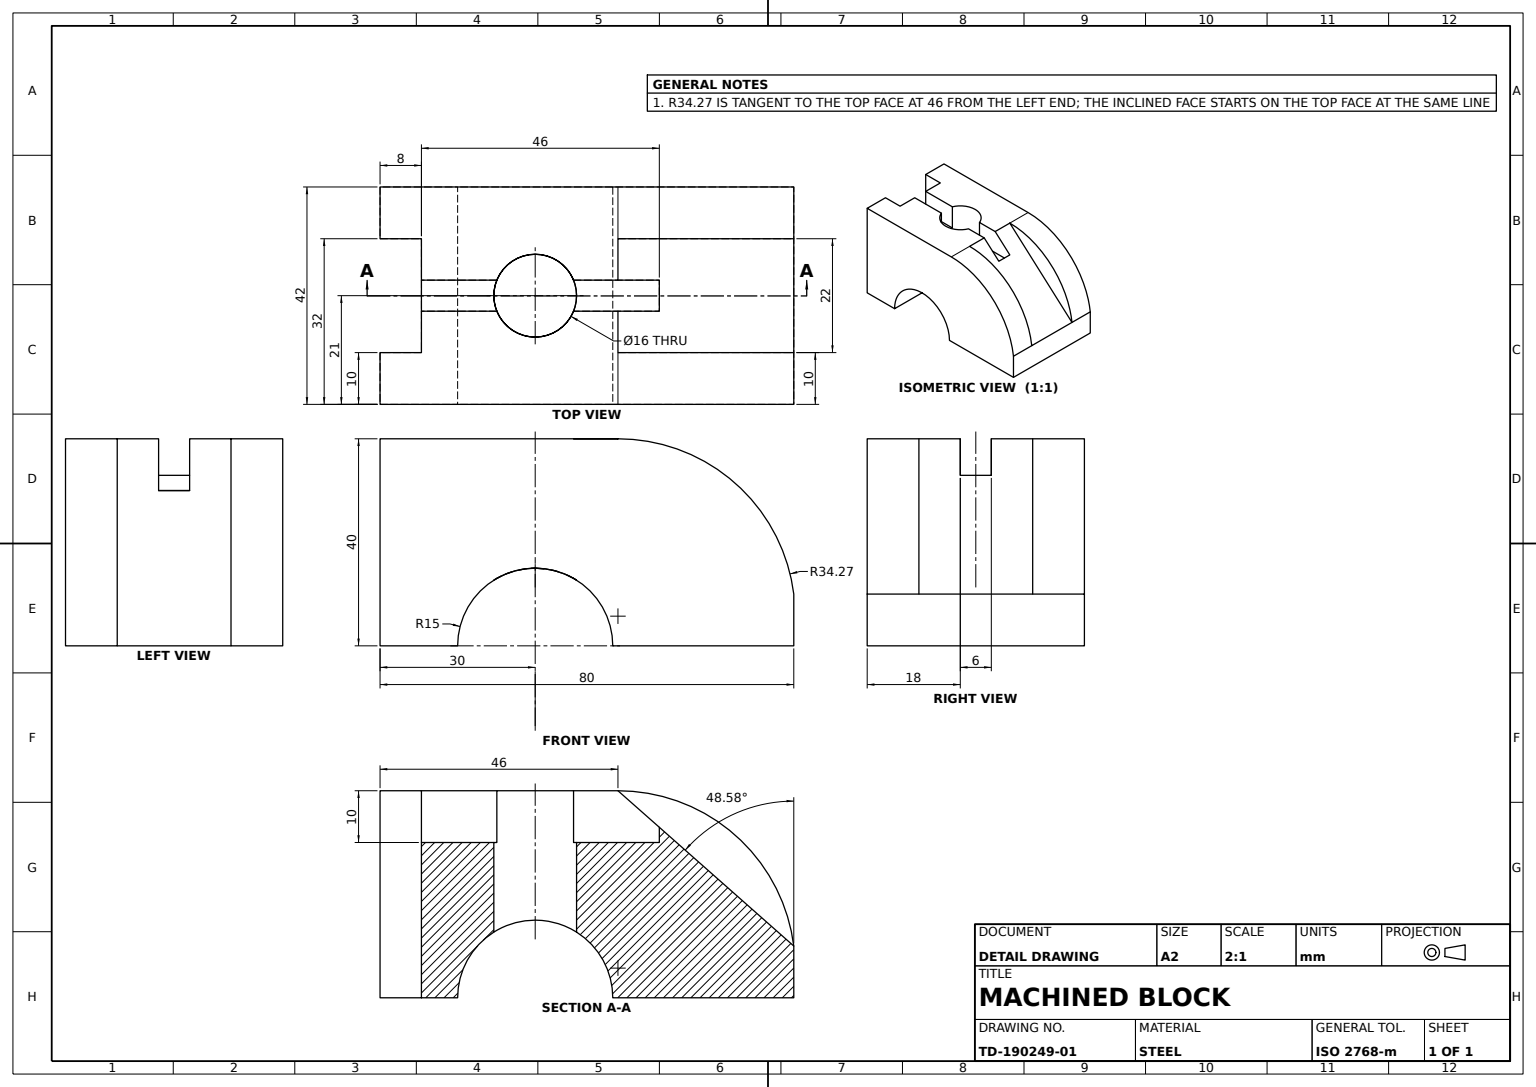
SolidWorks part; units mm, degrees
material "Plain Carbon Steel"
ref_plane "Front Plane" through (0, 0, 0) normal (0, 0, 1) x (1, 0, 0)
ref_plane "Top Plane" through (0, 0, 0) normal (0, 1, 0) x (1, 0, 0)
ref_plane "Right Plane" through (0, 0, 0) normal (1, 0, 0) x (0, 0, -1)
sketch "Base Block Profile" plane through (0, 0, 0) normal (0, 0, 1) x (1, 0, 0)
  line L0 (0, 0) -> (80, 0)
  line L1 (80, 0) -> (80, 40)
  line L2 (80, 40) -> (0, 40)
  line L3 (0, 40) -> (0, 0)
  dimension "D1" = 80
  dimension "D2" = 40
extrude "Base Block 80x40x42" add sketch "Base Block Profile" against normal blind 42
sketch "Top Slot Profile" plane through (0, 0, 0) normal (0, 0, 1) x (1, 0, 0)
  line L0 (0, 40) -> (0, 0) construction
  line L1 (46, 40) -> (46, 10)
  line L2 (80, 0) -> (80, 40) construction
  line L3 (46, 10) -> (80, 10)
  line L4 (0, 0) -> (80, 0) construction
  line L5 (80, 40) -> (0, 40) construction
  line L6 (46, 40) -> (80, 40)
  line L7 (80, 40) -> (80, 10)
  dimension "D1" = 46
  dimension "D2" = 10
extrude "Top Slot Cut 10" cut sketch "Top Slot Profile" against normal blind 10
sketch "Groove Profile" plane through (0, 0, -10) normal (0, 0, 1) x (1, 0, 0)
  line L0 (46, 40) -> (80, 10)
  line L1 (80, 10) -> (80, 40)
  line L2 (80, 40) -> (46, 40)
extrude "Groove Cut 22" cut sketch "Groove Profile" against normal blind 22
sketch "Groove Infill Profile" plane through (0, 0, 0) normal (0, 0, 1) x (1, 0, 0)
  line L0 (46, 40) -> (0, 40) construction
  line L1 (46, 40) -> (46, 10)
  line L2 (46, 10) -> (80, 10)
  arc A0 (46, 40) -> (80, 10) centre (46, 5.7333) cw
  dimension "D1" = 34.2667
extrude "Groove Infill Boss 10" add sketch "Groove Infill Profile" against normal blind 10
sketch "Groove Undercut Profile" plane through (0, 0, -32) normal (0, 0, 1) x (1, 0, 0)
  line L0 (46, 40) -> (80, 40)
  line L1 (80, 40) -> (80, 10)
  arc A0 (46, 40) -> (80, 10) centre (46, 5.7333) cw
  dimension "D1" = 34.2667
extrude "Groove Undercut 10" cut sketch "Groove Undercut Profile" against normal blind 10
sketch "Rounded End Profile" plane through (0, 0, 0) normal (0, 0, 1) x (1, 0, 0)
  line L0 (15, 0) -> (30, 0)
  line L1 (0, 0) -> (80, 0) construction
  line L2 (15, 0) -> (45, 0)
  line L3 (80, 0) -> (80, 10) construction
  arc A0 (45, 0) -> (15, 0) centre (30, 0) ccw
  line M5 (0, 0) -> (80, 0)
  dimension "D1" = 15
  dimension "D2" = 50
extrude "Rounded End Cut" cut sketch "Rounded End Profile" against normal blind 42 contours A0 M5
sketch "Arch Profile" plane through (0, 40, 0) normal (0, 1, 0) x (1, 0, 0)
  line L0 (0, 42) -> (8, 42)
  line L1 (46, 42) -> (0, 42) construction
  line L2 (46, 32) -> (46, 10) construction
  circle A0 centre (30, 21) radius 8
  dimension "D1" = 16
  dimension "D2" = 16
  dimension "D3" = 16
  dimension "D4" = 21
extrude "Arch Cut 10" cut sketch "Arch Profile" against normal blind 10 contours A0
sketch "Side Slot Profile" plane through (0, 0, 0) normal (-1, 0, 0) x (0, 0, 1)
  line L0 (-32, 40) -> (-10, 40)
  line L1 (-42, 40) -> (0, 40) construction
  line L2 (-32, 40) -> (-32, 0)
  line L3 (-42, 0) -> (0, 0) construction
  line L4 (-32, 0) -> (-10, 0)
  line L5 (-10, 0) -> (-10, 40)
  line L6 (0, 40) -> (0, 0) construction
  dimension "D1" = 10
  dimension "D2" = 32
extrude "Side Slot Cut 8" cut sketch "Side Slot Profile" against normal blind 8
sketch "Inclined Slot Profile" plane through (8, 0, 0) normal (-1, 0, 0) x (0, 0, 1)
  line L0 (-24, 40) -> (-18, 40)
  line L1 (-10, 40) -> (-32, 40) construction
  line L2 (-24, 40) -> (-24, 30)
  line L3 (-24, 30) -> (-18, 30)
  line L4 (-18, 30) -> (-18, 40)
  line L5 (-32, 40) -> (-32, 0) construction
  line L6 (-32, 0) -> (-10, 0) construction
  dimension "D1" = 8
  dimension "D2" = 14
  dimension "D3" = 30
extrude "Inclined Slot Cut 46" cut sketch "Inclined Slot Profile" against normal blind 46
sketch "Bore Ø16 Profile" plane through (0, 30, 0) normal (0, 1, 0) x (1, 0, 0)
  circle A0 centre (30, 21) radius 8
  dimension "D1" = 16
  dimension "D2" = 16
extrude "Bore Ø16 Cut 46" cut sketch "Bore Ø16 Profile" against normal blind 46
